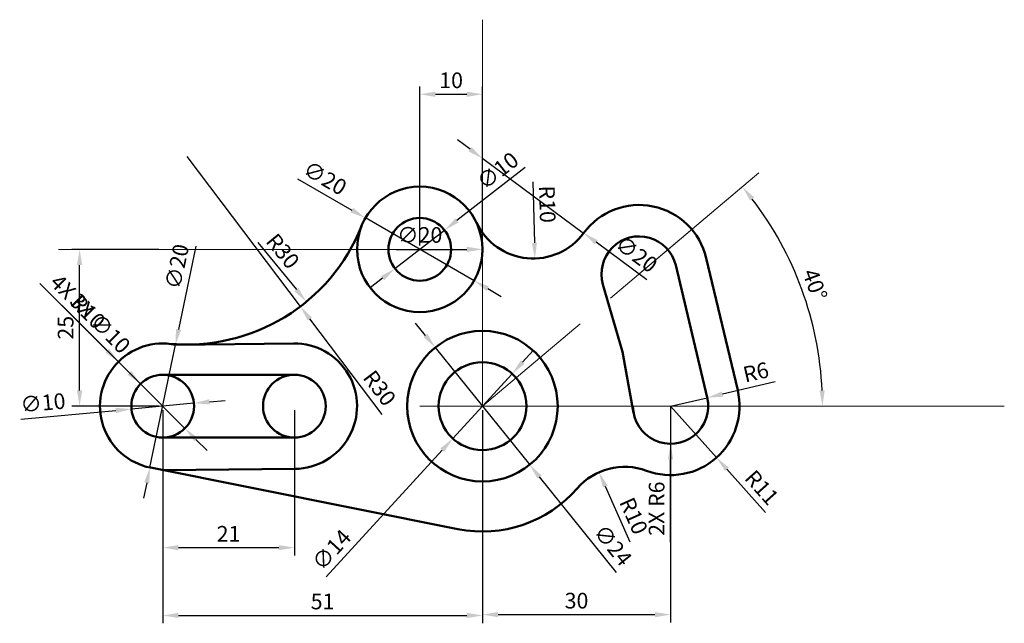
# Model space of a CAD drawing. Units: millimetres. Extents: x 2223 to 2380, y 1636 to 1732.
import ezdxf

# ---------------------------------------------------------------- set-up
doc = ezdxf.new("R2010")
doc.units = ezdxf.units.MM
for name, color, linetype, lineweight in [('M-CONS', 8, 'Continuous', 13), ('M-DIMS', 2, 'Continuous', 25), ('M-OUTL', 7, 'Continuous', 50)]:
    doc.layers.add(name, color=color, linetype=linetype, lineweight=lineweight)
doc.styles.get("Standard").update_dxf_attribs({"font": 'arial.ttf'})
doc.dimstyles.new('ISO-25', dxfattribs={"dimtxt": 2.5, "dimasz": 2.5, "dimexe": 1.25, "dimexo": 0.625, "dimtad": 1, "dimtxsty": 'Standard', "dimcen": 2.5, "dimadec": 0, "dimazin": 0, "dimtfac": 1, "dimtmove": 0, "dimatfit": 3, "dimfxl": 1, "dimarcsym": 0})

# ---------------------------------------------------------------- blocks, each defined once
blk = doc.blocks.new('*D1')
at = {"layer": 'Defpoints', "color": 0, "transparency": 16777216}
for p in [(2277.15, 1695.69), (2297.15, 1695.69)]:
    blk.add_point(p, dxfattribs=at)
at = {"layer": 'M-DIMS', "color": 0, "lineweight": -2, "transparency": 16777216}
blk.add_line((2283.38, 1695.69), (2294.65, 1695.69), dxfattribs=at)
at = {"layer": 'M-DIMS', "color": 0, "transparency": 16777216}
blk.add_solid([(2294.65, 1696.11), (2294.65, 1695.27), (2297.15, 1695.69)], dxfattribs=at)
at = {"layer": 'M-DIMS', "color": 0, "transparency": 16777216, "insert": (2287.15, 1697.66), "char_height": 2.5, "attachment_point": 5}
blk.add_mtext('∅20', dxfattribs=at)
blk = doc.blocks.new('*D2')
at = {"layer": 'Defpoints', "color": 0, "transparency": 16777216}
for p in [(2291.1, 1698.75), (2283.2, 1692.63)]:
    blk.add_point(p, dxfattribs=at)
at = {"layer": 'M-DIMS', "color": 0, "lineweight": -2, "transparency": 16777216}
for p, q in [((2303.96, 1708.73), (2293.08, 1700.29)), ((2283.2, 1692.63), (2291.1, 1698.75)), ((2281.22, 1691.09), (2279.25, 1689.56))]:
    blk.add_line(p, q, dxfattribs=at)
at = {"layer": 'M-DIMS', "color": 0, "transparency": 16777216}
for points in [[(2292.82, 1700.61), (2293.33, 1699.96), (2291.1, 1698.75)], [(2280.97, 1691.42), (2281.48, 1690.76), (2283.2, 1692.63)]]:
    blk.add_solid(points, dxfattribs=at)
at = {"layer": 'M-DIMS', "color": 0, "transparency": 16777216, "insert": (2299.77, 1707.97), "char_height": 2.5, "attachment_point": 5, "rotation": 37.7888}
blk.add_mtext('∅10', dxfattribs=at)
blk = doc.blocks.new('*D3')
at = {"layer": 'Defpoints', "color": 0, "transparency": 16777216}
for p in [(2297.19, 1710.16), (2313.29, 1698.29)]:
    blk.add_point(p, dxfattribs=at)
at = {"layer": 'M-DIMS', "color": 0, "lineweight": -2, "transparency": 16777216}
for p, q in [((2295.18, 1711.64), (2293.16, 1713.13)), ((2297.19, 1710.16), (2313.29, 1698.29)), ((2323.38, 1690.85), (2315.3, 1696.81))]:
    blk.add_line(p, q, dxfattribs=at)
at = {"layer": 'M-DIMS', "color": 0, "transparency": 16777216}
for points in [[(2295.42, 1711.98), (2294.93, 1711.31), (2297.19, 1710.16)], [(2315.55, 1697.14), (2315.05, 1696.47), (2313.29, 1698.29)]]:
    blk.add_solid(points, dxfattribs=at)
at = {"layer": 'M-DIMS', "color": 0, "transparency": 16777216, "insert": (2321.52, 1694.67), "char_height": 2.5, "attachment_point": 5, "rotation": 323.6024}
blk.add_mtext('∅20', dxfattribs=at)
blk = doc.blocks.new('*D4')
at = {"layer": 'Defpoints', "color": 0, "transparency": 16777216}
for p in [(2289.62, 1680.04), (2304.68, 1661.34)]:
    blk.add_point(p, dxfattribs=at)
at = {"layer": 'M-DIMS', "color": 0, "lineweight": -2, "transparency": 16777216}
for p, q in [((2288.05, 1681.98), (2286.49, 1683.93)), ((2289.62, 1680.04), (2304.68, 1661.34)), ((2318.54, 1644.14), (2306.25, 1659.4))]:
    blk.add_line(p, q, dxfattribs=at)
at = {"layer": 'M-DIMS', "color": 0, "transparency": 16777216}
for points in [[(2288.38, 1682.24), (2287.73, 1681.72), (2289.62, 1680.04)], [(2306.57, 1659.66), (2305.92, 1659.14), (2304.68, 1661.34)]]:
    blk.add_solid(points, dxfattribs=at)
at = {"layer": 'M-DIMS', "color": 0, "transparency": 16777216, "insert": (2317.71, 1648.31), "char_height": 2.5, "attachment_point": 5, "rotation": 308.8518}
blk.add_mtext('∅24', dxfattribs=at)
blk = doc.blocks.new('*D5')
at = {"layer": 'Defpoints', "color": 0, "transparency": 16777216}
for p in [(2301.88, 1675.85), (2292.43, 1665.53)]:
    blk.add_point(p, dxfattribs=at)
at = {"layer": 'M-DIMS', "color": 0, "lineweight": -2, "transparency": 16777216}
for p, q in [((2303.56, 1677.7), (2305.25, 1679.54)), ((2301.88, 1675.85), (2292.43, 1665.53)), ((2272.24, 1643.46), (2290.74, 1663.68))]:
    blk.add_line(p, q, dxfattribs=at)
at = {"layer": 'M-DIMS', "color": 0, "transparency": 16777216}
for points in [[(2303.26, 1677.98), (2303.87, 1677.42), (2301.88, 1675.85)], [(2290.43, 1663.96), (2291.05, 1663.4), (2292.43, 1665.53)]]:
    blk.add_solid(points, dxfattribs=at)
at = {"layer": 'M-DIMS', "color": 0, "transparency": 16777216, "insert": (2273.33, 1647.57), "char_height": 2.5, "attachment_point": 5, "rotation": 47.5468}
blk.add_mtext('∅14', dxfattribs=at)
blk = doc.blocks.new('*D6')
at = {"layer": 'Defpoints', "color": 0, "transparency": 16777216}
for p in [(2248.18, 1680.48), (2244.12, 1660.9)]:
    blk.add_point(p, dxfattribs=at)
at = {"layer": 'M-DIMS', "color": 0, "lineweight": -2, "transparency": 16777216}
for p, q in [((2251.44, 1696.18), (2248.69, 1682.93)), ((2244.12, 1660.9), (2248.18, 1680.48)), ((2243.61, 1658.45), (2243.1, 1656))]:
    blk.add_line(p, q, dxfattribs=at)
at = {"layer": 'M-DIMS', "color": 0, "transparency": 16777216}
for points in [[(2248.28, 1683.01), (2249.1, 1682.84), (2248.18, 1680.48)], [(2243.2, 1658.54), (2244.02, 1658.37), (2244.12, 1660.9)]]:
    blk.add_solid(points, dxfattribs=at)
at = {"layer": 'M-DIMS', "color": 0, "transparency": 16777216, "insert": (2248.74, 1692.89), "char_height": 2.5, "attachment_point": 5, "rotation": 78.2778}
blk.add_mtext('∅20', dxfattribs=at)
blk = doc.blocks.new('*D7')
at = {"layer": 'Defpoints', "color": 0, "transparency": 16777216}
for p in [(2251.13, 1671.15), (2241.17, 1670.23)]:
    blk.add_point(p, dxfattribs=at)
at = {"layer": 'M-DIMS', "color": 0, "lineweight": -2, "transparency": 16777216}
for p, q in [((2251.13, 1671.15), (2241.17, 1670.23)), ((2253.62, 1671.38), (2256.11, 1671.61)), ((2223.51, 1668.6), (2238.68, 1670))]:
    blk.add_line(p, q, dxfattribs=at)
at = {"layer": 'M-DIMS', "color": 0, "transparency": 16777216}
for points in [[(2253.58, 1671.79), (2253.66, 1670.97), (2251.13, 1671.15)], [(2238.64, 1670.41), (2238.72, 1669.58), (2241.17, 1670.23)]]:
    blk.add_solid(points, dxfattribs=at)
at = {"layer": 'M-DIMS', "color": 0, "transparency": 16777216, "insert": (2227.08, 1670.91), "char_height": 2.5, "attachment_point": 5, "rotation": 5.2797}
blk.add_mtext('∅10', dxfattribs=at)
blk = doc.blocks.new('*D8')
at = {"layer": 'Defpoints', "color": 0, "transparency": 16777216}
for p in [(2333, 1672.04), (2327.15, 1670.69)]:
    blk.add_point(p, dxfattribs=at)
at = {"layer": 'M-DIMS', "color": 0, "lineweight": -2, "transparency": 16777216}
for p, q in [((2343.83, 1674.54), (2335.43, 1672.6)), ((2327.15, 1670.69), (2333, 1672.04))]:
    blk.add_line(p, q, dxfattribs=at)
at = {"layer": 'M-DIMS', "color": 0, "transparency": 16777216}
blk.add_solid([(2335.34, 1673.01), (2335.53, 1672.2), (2333, 1672.04)], dxfattribs=at)
at = {"layer": 'M-DIMS', "color": 0, "transparency": 16777216, "insert": (2340.83, 1675.8), "char_height": 2.5, "attachment_point": 5, "rotation": 13.0035}
blk.add_mtext('R6', dxfattribs=at)
blk = doc.blocks.new('*D9')
at = {"layer": 'Defpoints', "color": 0, "transparency": 16777216}
for p in [(2327.15, 1670.69), (2334.48, 1662.49)]:
    blk.add_point(p, dxfattribs=at)
at = {"layer": 'M-DIMS', "color": 0, "lineweight": -2, "transparency": 16777216}
for p, q in [((2327.15, 1670.69), (2334.48, 1662.49)), ((2342.3, 1653.73), (2336.14, 1660.62))]:
    blk.add_line(p, q, dxfattribs=at)
at = {"layer": 'M-DIMS', "color": 0, "transparency": 16777216}
blk.add_solid([(2336.45, 1660.9), (2335.83, 1660.34), (2334.48, 1662.49)], dxfattribs=at)
at = {"layer": 'M-DIMS', "color": 0, "transparency": 16777216, "insert": (2341.46, 1657.5), "char_height": 2.5, "attachment_point": 5, "rotation": 311.7701}
blk.add_mtext('R11', dxfattribs=at)
blk = doc.blocks.new('*D10')
at = {"layer": 'Defpoints', "color": 0, "transparency": 16777216}
for p in [(2305.24, 1704.23), (2305.5, 1694.23)]:
    blk.add_point(p, dxfattribs=at)
at = {"layer": 'M-DIMS', "color": 0, "lineweight": -2, "transparency": 16777216}
blk.add_line((2305.18, 1706.44), (2305.44, 1696.73), dxfattribs=at)
at = {"layer": 'M-DIMS', "color": 0, "transparency": 16777216}
blk.add_solid([(2305.85, 1696.74), (2305.02, 1696.72), (2305.5, 1694.23)], dxfattribs=at)
at = {"layer": 'M-DIMS', "color": 0, "transparency": 16777216, "insert": (2307.17, 1702.88), "char_height": 2.5, "attachment_point": 5, "rotation": 271.5117}
blk.add_mtext('R10', dxfattribs=at)
blk = doc.blocks.new('*D11')
at = {"layer": 'Defpoints', "color": 0, "transparency": 16777216}
for p in [(2315.73, 1660.15), (2319.8, 1651.02)]:
    blk.add_point(p, dxfattribs=at)
at = {"layer": 'M-DIMS', "color": 0, "lineweight": -2, "transparency": 16777216}
blk.add_line((2320.7, 1649), (2316.75, 1657.87), dxfattribs=at)
at = {"layer": 'M-DIMS', "color": 0, "transparency": 16777216}
blk.add_solid([(2317.13, 1658.04), (2316.36, 1657.7), (2315.73, 1660.15)], dxfattribs=at)
at = {"layer": 'M-DIMS', "color": 0, "transparency": 16777216, "insert": (2320.97, 1653.06), "char_height": 2.5, "attachment_point": 5, "rotation": 294.0403}
blk.add_mtext('R10', dxfattribs=at)
blk = doc.blocks.new('*D12')
at = {"layer": 'Defpoints', "color": 0, "transparency": 16777216}
for p in [(2250, 1710.5), (2269.06, 1687.34)]:
    blk.add_point(p, dxfattribs=at)
at = {"layer": 'M-DIMS', "color": 0, "lineweight": -2, "transparency": 16777216}
blk.add_line((2261.3, 1696.77), (2267.47, 1689.27), dxfattribs=at)
at = {"layer": 'M-DIMS', "color": 0, "transparency": 16777216}
blk.add_solid([(2267.79, 1689.54), (2267.15, 1689.01), (2269.06, 1687.34)], dxfattribs=at)
at = {"layer": 'M-DIMS', "color": 0, "transparency": 16777216, "insert": (2265.06, 1695.2), "char_height": 2.5, "attachment_point": 5, "rotation": 309.4547}
blk.add_mtext('R30', dxfattribs=at)
blk = doc.blocks.new('*D13')
at = {"layer": 'Defpoints', "color": 0, "transparency": 16777216}
for p in [(2246.15, 1670.69), (2297.15, 1670.69), (2297.15, 1637.31)]:
    blk.add_point(p, dxfattribs=at)
at = {"layer": 'M-DIMS', "color": 0, "lineweight": -2, "transparency": 16777216}
for p, q in [((2246.15, 1670.06), (2246.15, 1636.06)), ((2297.15, 1670.06), (2297.15, 1636.06)), ((2248.65, 1637.31), (2294.65, 1637.31))]:
    blk.add_line(p, q, dxfattribs=at)
at = {"layer": 'M-DIMS', "color": 0, "transparency": 16777216}
for points in [[(2248.65, 1637.73), (2248.65, 1636.9), (2246.15, 1637.31)], [(2294.65, 1637.73), (2294.65, 1636.9), (2297.15, 1637.31)]]:
    blk.add_solid(points, dxfattribs=at)
at = {"layer": 'M-DIMS', "color": 0, "transparency": 16777216, "insert": (2271.65, 1639.22), "char_height": 2.5, "attachment_point": 5}
blk.add_mtext('51', dxfattribs=at)
blk = doc.blocks.new('*D14')
at = {"layer": 'Defpoints', "color": 0, "transparency": 16777216}
for p in [(2297.15, 1670.69), (2327.15, 1670.69), (2327.15, 1637.45)]:
    blk.add_point(p, dxfattribs=at)
at = {"layer": 'M-DIMS', "color": 0, "lineweight": -2, "transparency": 16777216}
for p, q in [((2297.15, 1670.06), (2297.15, 1636.2)), ((2327.15, 1670.06), (2327.15, 1636.2)), ((2299.65, 1637.45), (2324.65, 1637.45))]:
    blk.add_line(p, q, dxfattribs=at)
at = {"layer": 'M-DIMS', "color": 0, "transparency": 16777216}
for points in [[(2299.65, 1637.87), (2299.65, 1637.03), (2297.15, 1637.45)], [(2324.65, 1637.87), (2324.65, 1637.03), (2327.15, 1637.45)]]:
    blk.add_solid(points, dxfattribs=at)
at = {"layer": 'M-DIMS', "color": 0, "transparency": 16777216, "insert": (2312.15, 1639.35), "char_height": 2.5, "attachment_point": 5}
blk.add_mtext('30', dxfattribs=at)
blk = doc.blocks.new('*D15')
at = {"layer": 'Defpoints', "color": 0, "transparency": 16777216}
for p in [(2246.15, 1670.69), (2267.15, 1670.69), (2267.15, 1648.13)]:
    blk.add_point(p, dxfattribs=at)
at = {"layer": 'M-DIMS', "color": 0, "lineweight": -2, "transparency": 16777216}
for p, q in [((2246.15, 1670.06), (2246.15, 1646.88)), ((2267.15, 1670.06), (2267.15, 1646.88)), ((2248.65, 1648.13), (2264.65, 1648.13))]:
    blk.add_line(p, q, dxfattribs=at)
at = {"layer": 'M-DIMS', "color": 0, "transparency": 16777216}
for points in [[(2248.65, 1648.54), (2248.65, 1647.71), (2246.15, 1648.13)], [(2264.65, 1648.54), (2264.65, 1647.71), (2267.15, 1648.13)]]:
    blk.add_solid(points, dxfattribs=at)
at = {"layer": 'M-DIMS', "color": 0, "transparency": 16777216, "insert": (2256.65, 1650.01), "char_height": 2.5, "attachment_point": 5}
blk.add_mtext('21', dxfattribs=at)
blk = doc.blocks.new('*D16')
at = {"layer": 'Defpoints', "color": 0, "transparency": 16777216}
for p in [(2232.9, 1695.69), (2246.15, 1695.69), (2246.15, 1670.69)]:
    blk.add_point(p, dxfattribs=at)
at = {"layer": 'M-DIMS', "color": 0, "lineweight": -2, "transparency": 16777216}
for p, q in [((2245.53, 1695.69), (2231.65, 1695.69)), ((2232.9, 1673.19), (2232.9, 1693.19)), ((2245.53, 1670.69), (2231.65, 1670.69))]:
    blk.add_line(p, q, dxfattribs=at)
at = {"layer": 'M-DIMS', "color": 0, "transparency": 16777216}
for points in [[(2232.48, 1693.19), (2233.32, 1693.19), (2232.9, 1695.69)], [(2232.48, 1673.19), (2233.32, 1673.19), (2232.9, 1670.69)]]:
    blk.add_solid(points, dxfattribs=at)
at = {"layer": 'M-DIMS', "color": 0, "transparency": 16777216, "insert": (2231, 1683.19), "char_height": 2.5, "attachment_point": 5, "rotation": 90}
blk.add_mtext('25', dxfattribs=at)
blk = doc.blocks.new('*D17')
at = {"layer": 'Defpoints', "color": 0, "transparency": 16777216}
for p in [(2297.15, 1720.42), (2287.15, 1695.69), (2297.15, 1695.69)]:
    blk.add_point(p, dxfattribs=at)
at = {"layer": 'M-DIMS', "color": 0, "lineweight": -2, "transparency": 16777216}
for p, q in [((2287.15, 1696.31), (2287.15, 1721.67)), ((2297.15, 1696.31), (2297.15, 1721.67)), ((2289.65, 1720.42), (2294.65, 1720.42))]:
    blk.add_line(p, q, dxfattribs=at)
at = {"layer": 'M-DIMS', "color": 0, "transparency": 16777216}
for points in [[(2289.65, 1720.84), (2289.65, 1720), (2287.15, 1720.42)], [(2294.65, 1720.84), (2294.65, 1720), (2297.15, 1720.42)]]:
    blk.add_solid(points, dxfattribs=at)
at = {"layer": 'M-DIMS', "color": 0, "transparency": 16777216, "insert": (2292.15, 1722.32), "char_height": 2.5, "attachment_point": 5}
blk.add_mtext('10', dxfattribs=at)
blk = doc.blocks.new('*D18')
at = {"layer": 'Defpoints', "color": 0, "transparency": 16777216}
for p in [(2341.25, 1707.88), (2322.14, 1691.77), (2349.91, 1683.24), (2297.15, 1670.69), (2380.38, 1670.69)]:
    blk.add_point(p, dxfattribs=at)
at = {"layer": 'M-DIMS', "color": 0, "lineweight": -2, "transparency": 16777216}
blk.add_arc((2297.15, 1670.69), 54.23, 2.6414, 37.5012, dxfattribs=at)
at = {"layer": 'M-DIMS', "color": 0, "transparency": 16777216}
for points in [[(2339.85, 1703.44), (2340.5, 1703.97), (2338.61, 1705.65)], [(2351.74, 1673.2), (2350.91, 1673.18), (2351.38, 1670.69)]]:
    blk.add_solid(points, dxfattribs=at)
at = {"layer": 'M-DIMS', "color": 0, "transparency": 16777216, "insert": (2349.88, 1689.95), "char_height": 2.5, "attachment_point": 5, "rotation": 290.0713}
blk.add_mtext('40°', dxfattribs=at)
blk = doc.blocks.new('*D19')
at = {"layer": 'Defpoints', "color": 0, "transparency": 16777216}
for p in [(2250, 1710.5), (2268.1, 1686.58)]:
    blk.add_point(p, dxfattribs=at)
at = {"layer": 'M-DIMS', "color": 0, "lineweight": -2, "transparency": 16777216}
for p, q in [((2250, 1710.5), (2268.1, 1686.58)), ((2281.14, 1669.35), (2269.61, 1684.59))]:
    blk.add_line(p, q, dxfattribs=at)
at = {"layer": 'M-DIMS', "color": 0, "transparency": 16777216}
blk.add_solid([(2269.94, 1684.84), (2269.28, 1684.34), (2268.1, 1686.58)], dxfattribs=at)
at = {"layer": 'M-DIMS', "color": 0, "transparency": 16777216, "insert": (2280.48, 1673.38), "char_height": 2.5, "attachment_point": 5, "rotation": 307.1171}
blk.add_mtext('R30', dxfattribs=at)
blk = doc.blocks.new('*D20')
at = {"layer": 'Defpoints', "color": 0, "transparency": 16777216}
for p in [(2239.08, 1677.76), (2246.15, 1670.69)]:
    blk.add_point(p, dxfattribs=at)
at = {"layer": 'M-DIMS', "color": 0, "lineweight": -2, "transparency": 16777216}
for p, q in [((2226.57, 1690.27), (2237.31, 1679.53)), ((2246.15, 1670.69), (2239.08, 1677.76))]:
    blk.add_line(p, q, dxfattribs=at)
at = {"layer": 'M-DIMS', "color": 0, "transparency": 16777216}
blk.add_solid([(2237.61, 1679.82), (2237.02, 1679.23), (2239.08, 1677.76)], dxfattribs=at)
at = {"layer": 'M-DIMS', "color": 0, "transparency": 16777216, "insert": (2232.4, 1687.13), "char_height": 2.5, "attachment_point": 5, "rotation": 315.0019}
blk.add_mtext('4X R10', dxfattribs=at)
blk = doc.blocks.new('*D21')
at = {"layer": 'Defpoints', "color": 0, "transparency": 16777216}
for p in [(2327.15, 1670.69), (2327.15, 1664.69)]:
    blk.add_point(p, dxfattribs=at)
at = {"layer": 'M-DIMS', "color": 0, "lineweight": -2, "transparency": 16777216}
for p, q in [((2327.15, 1670.69), (2327.15, 1664.69)), ((2327.15, 1649), (2327.15, 1662.19))]:
    blk.add_line(p, q, dxfattribs=at)
at = {"layer": 'M-DIMS', "color": 0, "transparency": 16777216}
blk.add_solid([(2326.73, 1662.19), (2327.57, 1662.19), (2327.15, 1664.69)], dxfattribs=at)
at = {"layer": 'M-DIMS', "color": 0, "transparency": 16777216, "insert": (2325.25, 1654.34), "char_height": 2.5, "attachment_point": 5, "rotation": 89.9938}
blk.add_mtext('2X R6', dxfattribs=at)
blk = doc.blocks.new('*D22')
at = {"layer": 'Defpoints', "color": 0, "transparency": 16777216}
for p in [(2242.61, 1674.23), (2249.69, 1667.15)]:
    blk.add_point(p, dxfattribs=at)
at = {"layer": 'M-DIMS', "color": 0, "lineweight": -2, "transparency": 16777216}
for p, q in [((2230.04, 1686.8), (2240.85, 1675.99)), ((2249.69, 1667.15), (2242.61, 1674.23)), ((2251.45, 1665.39), (2253.22, 1663.62))]:
    blk.add_line(p, q, dxfattribs=at)
at = {"layer": 'M-DIMS', "color": 0, "transparency": 16777216}
for points in [[(2241.14, 1676.29), (2240.55, 1675.7), (2242.61, 1674.23)], [(2251.75, 1665.68), (2251.16, 1665.09), (2249.69, 1667.15)]]:
    blk.add_solid(points, dxfattribs=at)
at = {"layer": 'M-DIMS', "color": 0, "transparency": 16777216, "insert": (2235.95, 1683.67), "char_height": 2.5, "attachment_point": 5, "rotation": 315.0038}
blk.add_mtext('3X ∅10', dxfattribs=at)
blk = doc.blocks.new('*D23')
at = {"layer": 'Defpoints', "color": 0, "transparency": 16777216}
for p in [(2278.49, 1700.69), (2295.81, 1690.69)]:
    blk.add_point(p, dxfattribs=at)
at = {"layer": 'M-DIMS', "color": 0, "lineweight": -2, "transparency": 16777216}
for p, q in [((2267.63, 1706.96), (2276.33, 1701.94)), ((2295.81, 1690.69), (2278.49, 1700.69)), ((2297.98, 1689.44), (2300.14, 1688.19))]:
    blk.add_line(p, q, dxfattribs=at)
at = {"layer": 'M-DIMS', "color": 0, "transparency": 16777216}
for points in [[(2276.53, 1702.3), (2276.12, 1701.58), (2278.49, 1700.69)], [(2298.18, 1689.8), (2297.77, 1689.08), (2295.81, 1690.69)]]:
    blk.add_solid(points, dxfattribs=at)
at = {"layer": 'M-DIMS', "color": 0, "transparency": 16777216, "insert": (2271.88, 1706.78), "char_height": 2.5, "attachment_point": 5, "rotation": 330.0002}
blk.add_mtext('∅20', dxfattribs=at)

msp = doc.modelspace()

# ---------------------------------------------------------------- linework, layer by layer
at = {"layer": 'M-CONS'}
for p, q in [((2297.151, 1670.69), (2297.151, 1732.309)), ((2317.554, 1687.897), (2341.252, 1707.882)), ((2341.252, 1707.882), (2322.141, 1691.765)), ((2341.252, 1707.882), (2341.252, 1707.882)), ((2287.151, 1695.69), (2229.557, 1695.69)), ((2297.151, 1670.69), (2312.722, 1683.822)), ((2297.151, 1670.69), (2287.151, 1670.69)), ((2297.151, 1670.69), (2380.376, 1670.69)), ((2327.151, 1670.69), (2327.151, 1665.211))]:
    msp.add_line(p, q, dxfattribs=at)
at = {"layer": 'M-OUTL'}
for p, q in [((2327.978, 1693.153), (2332.988, 1672.077)), ((2332.842, 1694.309), (2337.852, 1673.234)), ((2316.373, 1690.112), (2319.459, 1679.347)), ((2248.182, 1680.481), (2267.04, 1680.689)), ((2319.459, 1679.347), (2321.249, 1669.605)), ((2267.151, 1675.69), (2246.151, 1675.69)), ((2267.151, 1665.69), (2246.151, 1665.69)), ((2244.19, 1660.884), (2293.229, 1651.078)), ((2246.151, 1660.492), (2267.245, 1660.69))]:
    msp.add_line(p, q, dxfattribs=at)
for centre, radius in [((2287.151, 1695.69), 10), ((2287.151, 1695.69), 5), ((2297.151, 1670.69), 12), ((2297.151, 1670.69), 7), ((2246.151, 1670.69), 5), ((2267.151, 1670.69), 5)]:
    msp.add_circle(centre, radius, dxfattribs=at)
for centre, radius, start, end in [((2322.141, 1691.765), 11, 13.37205, 143.60236), ((2249.995, 1710.505), 30, 264.48446, 338.26155), ((2305.237, 1704.226), 10, 205.26587, 323.60236), ((2322.141, 1691.765), 6, 13.37205, 195.99752), ((2246.151, 1670.69), 10, 78.2778, 258.69227), ((2267.151, 1670.69), 10, 270.53889, 90.63178), ((2327.151, 1670.69), 11, 249.51268, 13.37205), ((2327.151, 1670.69), 6, 180, 13.37205), ((2319.801, 1651.018), 10, 69.51268, 139.02537), ((2297.151, 1670.69), 20, 258.69227, 319.02537)]:
    msp.add_arc(centre, radius, start, end, dxfattribs=at)

# ---------------------------------------------------------------- dimensions: what is measured, and where the dimension line sits
at = {"layer": 'M-DIMS'}
for p1, p2, distance, picture, middle in [((2287.151, 1695.69), (2297.151, 1695.69), 24.731, '*D17', (2292.151, 1722.322)), ((2246.151, 1670.69), (2246.151, 1695.69), 13.252, '*D16', (2230.997, 1683.19)), ((2246.151, 1670.69), (2297.151, 1670.69), -33.376, '*D13', (2271.651, 1639.215)), ((2246.151, 1670.69), (2267.151, 1670.69), -22.563, '*D15', (2256.651, 1650.007)), ((2297.151, 1670.69), (2327.151, 1670.69), -33.24, '*D14', (2312.151, 1639.352))]:
    dim = msp.add_aligned_dim(p1=p1, p2=p2, distance=distance, dimstyle='ISO-25', override={"dimclrd": 0, "dimclre": 0, "dimclrt": 0}, dxfattribs=at)
    dim.commit()
    dim.dimension.update_dxf_attribs({"geometry": picture, "text_midpoint": middle})
for p1, p2, override, picture, middle in [((2297.188, 1710.16), (2313.287, 1698.292), {"dimclrd": 0, "dimclre": 0, "dimclrt": 0}, '*D3', (2321.517, 1694.674)), ((2295.811, 1690.69), (2278.49, 1700.69), {"dimdec": 0, "dimlfac": 1, "dimrnd": 0, "dimzin": 0, "dimdsep": 46, "dimlunit": 2}, '*D23', (2270.894, 1705.075))]:
    dim = msp.add_diameter_dim_2p(p1=p1, p2=p2, dimstyle='ISO-25', override=override, dxfattribs=at)
    dim.commit()
    dim.dimension.update_dxf_attribs({"geometry": picture, "text_midpoint": middle})
for center, mpoint, override, picture, middle in [((2249.995, 1710.505), (2269.059, 1687.341), {"dimclrd": 0, "dimclre": 0, "dimclrt": 0}, '*D12', (2263.589, 1693.987)), ((2249.995, 1710.505), (2268.099, 1686.583), {"dimdec": 0, "dimlfac": 1, "dimrnd": 0, "dimzin": 0, "dimdsep": 46, "dimlunit": 2}, '*D19', (2278.961, 1672.229)), ((2305.237, 1704.226), (2305.501, 1694.23), {"dimclrd": 0, "dimclre": 0, "dimclrt": 0}, '*D10', (2305.274, 1702.834)), ((2327.151, 1670.69), (2332.997, 1672.04), {"dimclrd": 0, "dimclre": 0, "dimclrt": 0}, '*D8', (2341.26, 1673.948)), ((2319.801, 1651.018), (2315.727, 1660.151), {"dimclrd": 0, "dimclre": 0, "dimclrt": 0}, '*D11', (2319.233, 1652.29))]:
    dim = msp.add_radius_dim(center=center, mpoint=mpoint, dimstyle='ISO-25', override=override, dxfattribs=at)
    dim.commit()
    dim.dimension.update_dxf_attribs({"geometry": picture, "text_midpoint": middle, "dimtype": 164})
for p1, p2, picture, middle in [((2283.199, 1692.626), (2291.102, 1698.754), '*D2', (2300.982, 1706.414)), ((2277.151, 1695.69), (2297.151, 1695.69), '*D1', (2287.151, 1695.69)), ((2244.119, 1660.898), (2248.182, 1680.481), '*D6', (2250.673, 1692.485)), ((2289.623, 1680.035), (2304.678, 1661.345), '*D4', (2316.173, 1647.075)), ((2301.876, 1675.855), (2292.426, 1665.525), '*D5', (2274.782, 1646.239)), ((2251.129, 1671.15), (2241.172, 1670.23), '*D7', (2227.26, 1668.944))]:
    dim = msp.add_diameter_dim_2p(p1=p1, p2=p2, dimstyle='ISO-25', override={"dimclrd": 0, "dimclre": 0, "dimclrt": 0}, dxfattribs=at)
    dim.commit()
    dim.dimension.update_dxf_attribs({"geometry": picture, "text_midpoint": middle, "dimtype": 163})
dim = msp.add_angular_dim_2l(base=(2349.912, 1683.241), line1=((2297.151, 1670.69), (2380.376, 1670.69)), line2=((2341.252, 1707.882), (2322.141, 1691.765)), dimstyle='ISO-25', override={"dimclrd": 0, "dimclre": 0, "dimclrt": 0}, dxfattribs=at)
dim.commit()
dim.dimension.update_dxf_attribs({"geometry": '*D18', "text_midpoint": (2349.877, 1689.955)})
for center, mpoint, text, picture, middle in [((2246.151, 1670.69), (2239.079, 1677.761), '4X <>', '*D20', (2232.402, 1687.126)), ((2327.151, 1670.69), (2327.15, 1664.69), '2X <>', '*D21', (2325.247, 1654.343))]:
    dim = msp.add_radius_dim(center=center, mpoint=mpoint, text=text, dimstyle='ISO-25', override={"dimdec": 0, "dimlfac": 1, "dimrnd": 0, "dimzin": 0, "dimdsep": 46, "dimlunit": 2}, dxfattribs=at)
    dim.commit()
    dim.dimension.update_dxf_attribs({"geometry": picture, "text_midpoint": middle})
dim = msp.add_diameter_dim_2p(p1=(2249.686, 1667.155), p2=(2242.615, 1674.225), text='3X <>', dimstyle='ISO-25', override={"dimdec": 0, "dimlfac": 1, "dimrnd": 0, "dimzin": 0, "dimdsep": 46, "dimlunit": 2}, dxfattribs=at)
dim.commit()
dim.dimension.update_dxf_attribs({"geometry": '*D22', "text_midpoint": (2234.561, 1682.278)})
dim = msp.add_radius_dim(center=(2327.151, 1670.69), mpoint=(2334.478, 1662.486), dimstyle='ISO-25', override={"dimclrd": 0, "dimclre": 0, "dimclrt": 0}, dxfattribs=at)
dim.commit()
dim.dimension.update_dxf_attribs({"geometry": '*D9', "text_midpoint": (2341.456, 1657.495)})

doc.saveas('drawing.dxf')
